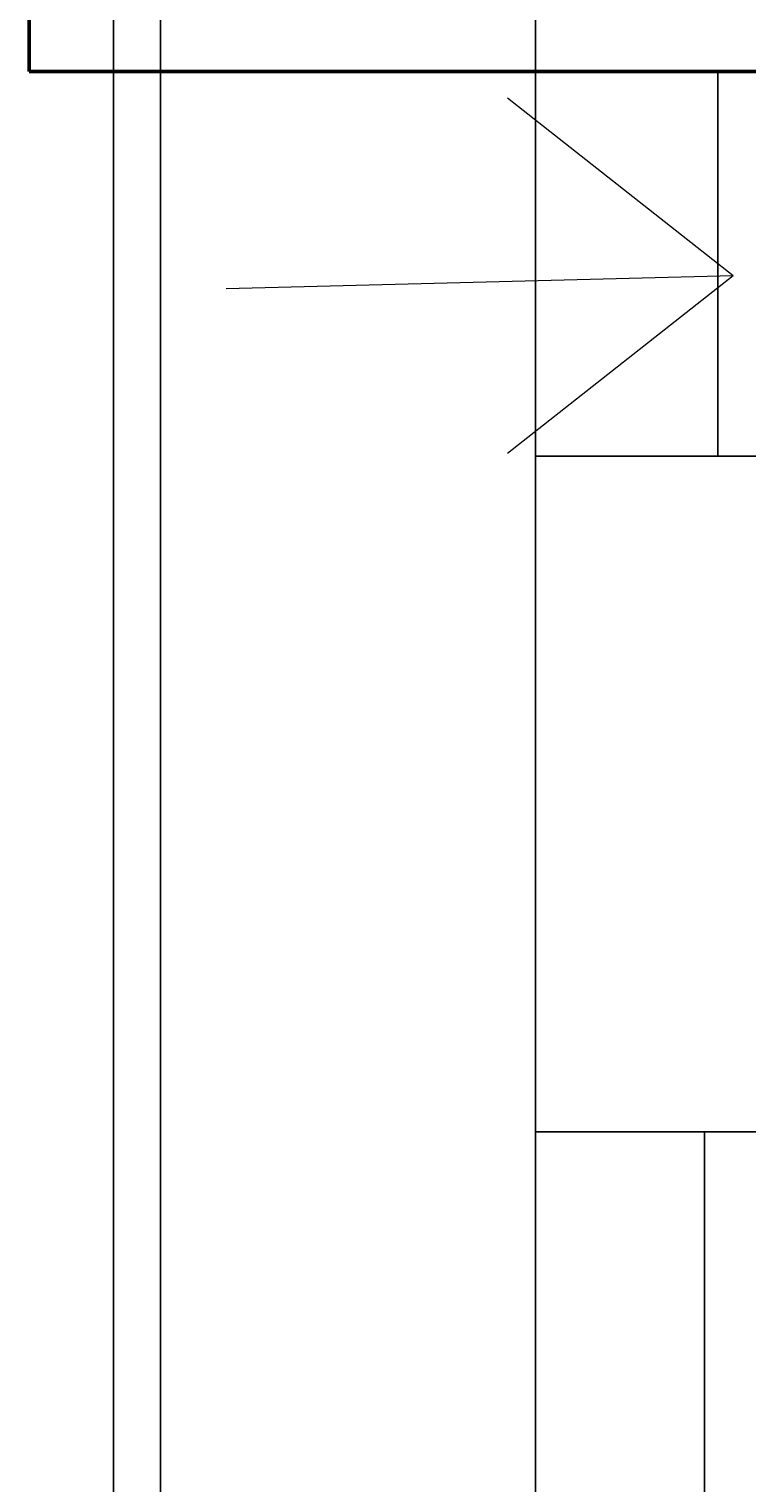
# Model space of a CAD drawing. Units: inches. Extents: x -364 to 705, y -52 to 1250.
# Tile 12 of 34: x 359 to 435, y 153 to 308. Entities that reach past the tile are written whole.
import ezdxf

# ---------------------------------------------------------------- set-up
doc = ezdxf.new("R2010")
doc.units = ezdxf.units.IN
doc.header["$MEASUREMENT"] = 0
for name, color, linetype, lineweight in [('A-ANNO-DIMS', 4, 'Continuous', 18), ('A-ANNO-SYMB', 7, 'Continuous', 18), ('A-FLOR-STRS', 7, 'Continuous', 25), ('A-WALL', 41, 'Continuous', 50)]:
    doc.layers.add(name, color=color, linetype=linetype, lineweight=lineweight)
doc.styles.get("Standard").update_dxf_attribs({"font": 'arial.ttf'})
doc.dimstyles.get("Standard").update_dxf_attribs({"dimtxt": 1, "dimasz": 1, "dimexe": 0.18, "dimexo": 0.0625, "dimgap": 0.09, "dimtad": 0, "dimtih": 1, "dimtoh": 1, "dimdec": 0, "dimzin": 0, "dimdsep": 46, "dimlunit": 3, "dimtxsty": 'Standard', "dimcen": 0.09, "dimadec": 0, "dimazin": 0, "dimtfac": 1, "dimtdec": 0, "dimtofl": 0, "dimtmove": 0, "dimatfit": 3, "dimfxl": 1, "dimtolj": 1, "dimtzin": 0, "dimarcsym": 0})

# ---------------------------------------------------------------- blocks, each defined once
blk = doc.blocks.new('STAIR-DIRECTION')
for q in [(0, 30), (20.33, 0), (37.87, 30)]:
    blk.add_line((18.93, 54.04), q)
blk = doc.blocks.new('*D101')
at = {"layer": 'A-ANNO-DIMS', "color": 0, "lineweight": -2, "transparency": 16777216}
for p, q in [((372.58, 408.05), (372.58, -51.32)), ((412.58, 408.05), (412.58, -51.32)), ((373.58, -51.14), (391.16, -51.14)), ((411.58, -51.14), (394, -51.14))]:
    blk.add_line(p, q, dxfattribs=at)
at = {"layer": 'A-ANNO-DIMS', "color": 0, "transparency": 16777216}
for points in [[(373.58, -50.97), (373.58, -51.3), (372.58, -51.14)], [(411.58, -50.97), (411.58, -51.3), (412.58, -51.14)]]:
    blk.add_solid(points, dxfattribs=at)
at = {"layer": 'Defpoints', "color": 0, "transparency": 16777216}
for p in [(372.58, 408.11), (412.58, 408.11), (412.58, -51.14)]:
    blk.add_point(p, dxfattribs=at)
at = {"layer": 'A-ANNO-DIMS', "color": 0, "transparency": 16777216, "insert": (392.58, -51.14), "char_height": 1, "attachment_point": 5}
blk.add_mtext('\\A1;3\'-4"', dxfattribs=at)
blk = doc.blocks.new('*D102')
at = {"layer": 'A-ANNO-DIMS', "color": 0, "lineweight": -2, "transparency": 16777216}
for p, q in [((367.58, 408.05), (367.58, -51.32)), ((372.58, 408.05), (372.58, -51.32)), ((366.58, -51.14), (365.58, -51.14)), ((373.58, -51.14), (374.58, -51.14))]:
    blk.add_line(p, q, dxfattribs=at)
at = {"layer": 'A-ANNO-DIMS', "color": 0, "transparency": 16777216}
for points in [[(366.58, -50.97), (366.58, -51.3), (367.58, -51.14)], [(373.58, -50.97), (373.58, -51.3), (372.58, -51.14)]]:
    blk.add_solid(points, dxfattribs=at)
at = {"layer": 'Defpoints', "color": 0, "transparency": 16777216}
for p in [(367.58, 408.11), (372.58, 408.11), (372.58, -51.14)]:
    blk.add_point(p, dxfattribs=at)
at = {"layer": 'A-ANNO-DIMS', "color": 0, "transparency": 16777216, "insert": (370.08, -51.14), "char_height": 1, "attachment_point": 5}
blk.add_mtext('\\A1;0\'-5"', dxfattribs=at)

msp = doc.modelspace()

# ---------------------------------------------------------------- linework, layer by layer
at = {"layer": 'A-FLOR-STRS'}
for p, q in [((432, 303.11), (432, 262.11)), ((412.58, 262.11), (468, 262.11)), ((412.58, 190.11), (538.58, 190.11)), ((430.58, 190.11), (430.58, 149.11))]:
    msp.add_line(p, q, dxfattribs=at)
at = {"layer": 'A-WALL'}
for p, q in [((358.58, 303.11), (358.58, 417.11)), ((538.58, 303.11), (358.58, 303.11))]:
    msp.add_line(p, q, dxfattribs=at)

# ---------------------------------------------------------------- block references
at = {"layer": 'A-ANNO-SYMB', "rotation": 269.9999999999998}
msp.add_blockref('STAIR-DIRECTION', (379.58, 300.27), dxfattribs=at)

# ---------------------------------------------------------------- dimensions: what is measured, and where the dimension line sits
at = {"layer": 'A-ANNO-DIMS'}
for base, p1, p2, picture, middle in [((372.58, -51.14), (367.58, 408.11), (372.58, 408.11), '*D102', (370.08, -51.14)), ((412.58, -51.14), (372.58, 408.11), (412.58, 408.11), '*D101', (392.58, -51.14))]:
    dim = msp.add_linear_dim(base=base, p1=p1, p2=p2, dimstyle='Standard', override={"dimdec": 1, "dimlfac": 1, "dimrnd": 0, "dimzin": 1, "dimdsep": 46, "dimlunit": 4, "dimfrac": 2}, dxfattribs=at)
    dim.commit()
    dim.dimension.update_dxf_attribs({"geometry": picture, "text_midpoint": middle})

doc.saveas('drawing.dxf')
